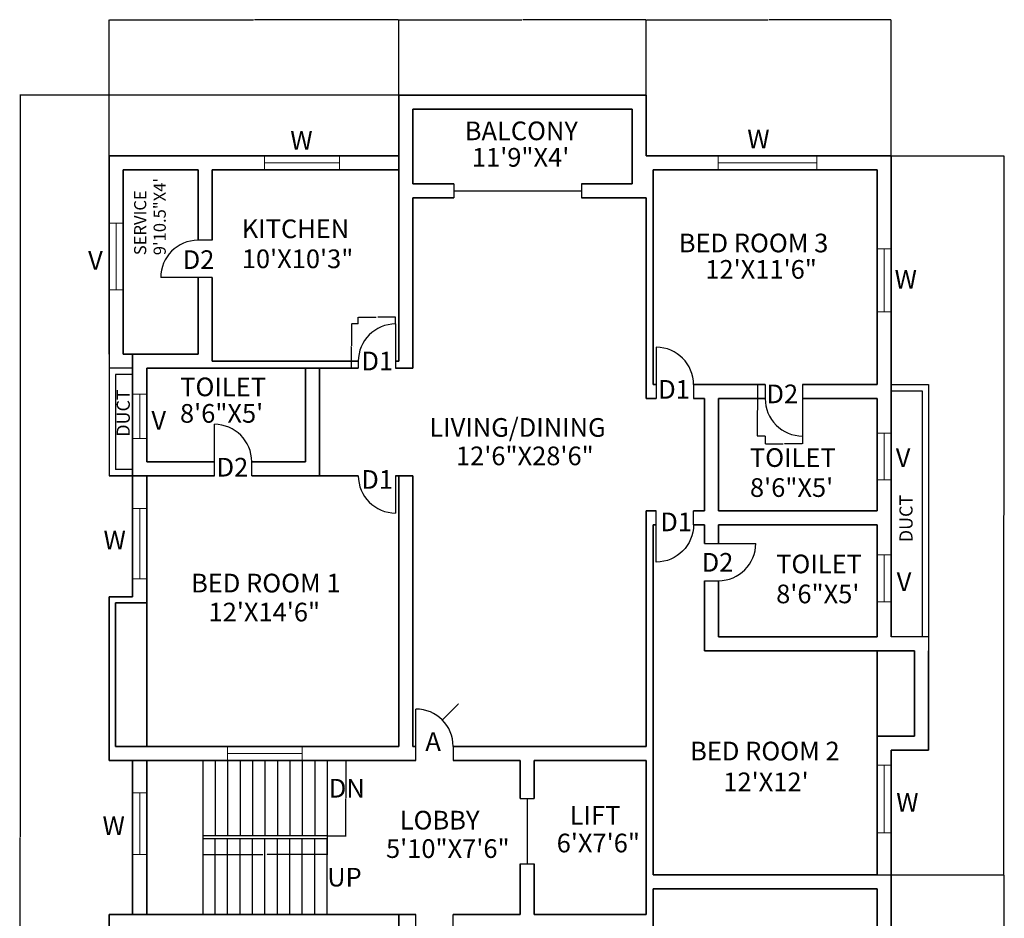
# Model space of a CAD drawing. Units: feet. Extents: x 48598101 to 48598734, y 135188346 to 135189397.
# Tile 2 of 2: x 48598101 to 48598734, y 135188819 to 135189397. Entities that reach past the tile are written whole.
import ezdxf

# ---------------------------------------------------------------- set-up
doc = ezdxf.new("R2010")
doc.units = ezdxf.units.FT
for name, color, linetype, lineweight in [('A-ANNO-DIMS', 2, 'Continuous', 18), ('A-ANNO-TEXT', 7, 'Continuous', 18), ('A-AREA-IDEN', 7, 'Continuous', 18), ('A-DOOR', 3, 'Continuous', 25), ('A-FLOR-SHFT', 7, 'Continuous', 25), ('A-FLOR-STRS', 7, 'Continuous', 25), ('A-GLAZ', 4, 'Continuous', 18), ('A-WALL', 7, 'Continuous', 35)]:
    doc.layers.add(name, color=color, linetype=linetype, lineweight=lineweight)
doc.styles.get("Standard").update_dxf_attribs({"font": 'arial.ttf'})
doc.dimstyles.get("Standard").update_dxf_attribs({"dimtxt": 0.18, "dimasz": 0.18, "dimexe": 0.18, "dimexo": 0.0625, "dimgap": 0.09, "dimtad": 0, "dimtih": 1, "dimtoh": 1, "dimdec": 4, "dimzin": 0, "dimdsep": 46, "dimtxsty": 'Standard', "dimcen": 0.09, "dimadec": 0, "dimazin": 0, "dimtfac": 1, "dimtdec": 4, "dimtofl": 0, "dimtmove": 0, "dimatfit": 3, "dimfxl": 1, "dimtolj": 1, "dimtzin": 0, "dimarcsym": 0})

# ---------------------------------------------------------------- blocks, each defined once
blk = doc.blocks.new('DOOR-D1-KITCHEN')
for p, q in [((24, 28.5), (24, 0)), ((0, 4.5), (0, 0))]:
    blk.add_line(p, q)
blk.add_arc((24, 4.5), 24, 90, 180)
blk = doc.blocks.new('DOOR-D1-BED-SWING')
blk.add_line((24, 24), (24, 0))
blk.add_arc((24, 24), 24, 180, 270)
blk = doc.blocks.new('DOOR-D1-BED-JAMB')
for p, q in [((0, 33), (0, 0)), ((24, 9), (24, 0))]:
    blk.add_line(p, q)
blk.add_arc((0, 9), 24, 0, 90)
blk = doc.blocks.new('DOOR-D2-SINGLE')
for p, q in [((33, 24), (24, 24)), ((33, 0), (0, 0))]:
    blk.add_line(p, q)
blk.add_arc((24, 0), 24, 90, 180)
blk = doc.blocks.new('STAIR-FLIGHT-10-TREAD')
for p, q in [((8, 48.5), (8, 0)), ((16, 48.5), (16, 0)), ((24, 48.5), (24, 0)), ((32, 48.5), (32, 0)), ((40, 48.5), (40, 0)), ((48, 48.5), (48, 0)), ((56, 48.5), (56, 0)), ((64, 48.5), (64, 0)), ((72, 48.5), (72, 0)), ((80, 48.5), (80, 0)), ((80, 0), (0, 0))]:
    blk.add_line(p, q)
blk = doc.blocks.new('SHAFT-VENT-NARROW')
for p, q in [((0, 78), (0, 0)), ((15, 69), (0, 69)), ((15, 65), (4, 65)), ((4, 65), (4, 4)), ((15, 4), (4, 4))]:
    blk.add_line(p, q)
blk = doc.blocks.new('*D7')
at = {"layer": 'A-ANNO-DIMS', "color": 0, "lineweight": -2, "transparency": 16777216}
for p, q in [((48598579.89, 135189162.29), (48598574.83, 135189162.29)), ((48598575.01, 135189162.11), (48598575.01, 135189145.97)), ((48598575.01, 135189129.47), (48598575.01, 135189145.61)), ((48598579.89, 135189129.29), (48598574.83, 135189129.29))]:
    blk.add_line(p, q, dxfattribs=at)
at = {"layer": 'A-ANNO-DIMS', "color": 0, "transparency": 16777216}
for points in [[(48598574.98, 135189162.11), (48598575.04, 135189162.11), (48598575.01, 135189162.29)], [(48598574.98, 135189129.47), (48598575.04, 135189129.47), (48598575.01, 135189129.29)]]:
    blk.add_solid(points, dxfattribs=at)
at = {"layer": 'Defpoints', "color": 0, "transparency": 16777216}
for p in [(48598575.01, 135189162.29), (48598579.96, 135189162.29), (48598579.96, 135189129.29)]:
    blk.add_point(p, dxfattribs=at)
at = {"layer": 'A-ANNO-DIMS', "color": 0, "transparency": 16777216, "insert": (48598575.01, 135189145.79), "char_height": 0.18, "attachment_point": 5}
blk.add_mtext('\\A1;D2 DOOR 33 TYP.', dxfattribs=at)
blk = doc.blocks.new('*D8')
at = {"layer": 'A-ANNO-DIMS', "color": 0, "lineweight": -2, "transparency": 16777216}
for p, q in [((48598579.96, 135189129.23), (48598579.96, 135189124.16)), ((48598603.96, 135189129.23), (48598603.96, 135189124.16)), ((48598580.14, 135189124.34), (48598591.43, 135189124.34)), ((48598603.78, 135189124.34), (48598592.49, 135189124.34))]:
    blk.add_line(p, q, dxfattribs=at)
at = {"layer": 'A-ANNO-DIMS', "color": 0, "transparency": 16777216}
for points in [[(48598580.14, 135189124.37), (48598580.14, 135189124.31), (48598579.96, 135189124.34)], [(48598603.78, 135189124.37), (48598603.78, 135189124.31), (48598603.96, 135189124.34)]]:
    blk.add_solid(points, dxfattribs=at)
at = {"layer": 'Defpoints', "color": 0, "transparency": 16777216}
for p in [(48598579.96, 135189129.29), (48598603.96, 135189129.29), (48598579.96, 135189124.34)]:
    blk.add_point(p, dxfattribs=at)
at = {"layer": 'A-ANNO-DIMS', "color": 0, "transparency": 16777216, "insert": (48598591.96, 135189124.34), "char_height": 0.18, "attachment_point": 5}
blk.add_mtext('\\A1;24 TYP.', dxfattribs=at)
blk = doc.blocks.new('*D11')
at = {"layer": 'A-ANNO-DIMS', "color": 0, "lineweight": -2, "transparency": 16777216}
for p, q in [((48598318.39, 135189201.29), (48598314, 135189201.29)), ((48598314.18, 135189201.11), (48598314.18, 135189187.22)), ((48598314.18, 135189172.97), (48598314.18, 135189186.86)), ((48598318.39, 135189172.79), (48598314, 135189172.79))]:
    blk.add_line(p, q, dxfattribs=at)
at = {"layer": 'A-ANNO-DIMS', "color": 0, "transparency": 16777216}
for points in [[(48598314.15, 135189201.11), (48598314.21, 135189201.11), (48598314.18, 135189201.29)], [(48598314.15, 135189172.97), (48598314.21, 135189172.97), (48598314.18, 135189172.79)]]:
    blk.add_solid(points, dxfattribs=at)
at = {"layer": 'Defpoints', "color": 0, "transparency": 16777216}
for p in [(48598314.18, 135189201.29), (48598318.46, 135189201.29), (48598318.46, 135189172.79)]:
    blk.add_point(p, dxfattribs=at)
at = {"layer": 'A-ANNO-DIMS', "color": 0, "transparency": 16777216, "insert": (48598314.18, 135189187.04), "char_height": 0.18, "attachment_point": 5}
blk.add_mtext('\\A1;D1 KITCHEN 29 TYP.', dxfattribs=at)
blk = doc.blocks.new('*D12')
at = {"layer": 'A-ANNO-DIMS', "color": 0, "lineweight": -2, "transparency": 16777216}
for p, q in [((48598318.46, 135189201.35), (48598318.46, 135189205.75)), ((48598318.64, 135189205.57), (48598329.93, 135189205.57)), ((48598342.28, 135189205.57), (48598330.99, 135189205.57)), ((48598342.46, 135189201.35), (48598342.46, 135189205.75))]:
    blk.add_line(p, q, dxfattribs=at)
at = {"layer": 'A-ANNO-DIMS', "color": 0, "transparency": 16777216}
for points in [[(48598318.64, 135189205.6), (48598318.64, 135189205.54), (48598318.46, 135189205.57)], [(48598342.28, 135189205.6), (48598342.28, 135189205.54), (48598342.46, 135189205.57)]]:
    blk.add_solid(points, dxfattribs=at)
at = {"layer": 'Defpoints', "color": 0, "transparency": 16777216}
for p in [(48598342.46, 135189205.57), (48598318.46, 135189201.29), (48598342.46, 135189201.29)]:
    blk.add_point(p, dxfattribs=at)
at = {"layer": 'A-ANNO-DIMS', "color": 0, "transparency": 16777216, "insert": (48598330.46, 135189205.57), "char_height": 0.18, "attachment_point": 5}
blk.add_mtext('\\A1;24 TYP.', dxfattribs=at)
blk = doc.blocks.new('*D15')
at = {"layer": 'A-ANNO-DIMS', "color": 0, "lineweight": -2, "transparency": 16777216}
for p, q in [((48598218.46, 135188872.23), (48598218.46, 135188860.11)), ((48598298.46, 135188872.23), (48598298.46, 135188860.11)), ((48598218.64, 135188860.29), (48598257.04, 135188860.29)), ((48598298.28, 135188860.29), (48598259.87, 135188860.29))]:
    blk.add_line(p, q, dxfattribs=at)
at = {"layer": 'A-ANNO-DIMS', "color": 0, "transparency": 16777216}
for points in [[(48598218.64, 135188860.32), (48598218.64, 135188860.26), (48598218.46, 135188860.29)], [(48598298.28, 135188860.32), (48598298.28, 135188860.26), (48598298.46, 135188860.29)]]:
    blk.add_solid(points, dxfattribs=at)
at = {"layer": 'Defpoints', "color": 0, "transparency": 16777216}
for p in [(48598218.46, 135188872.29), (48598298.46, 135188872.29), (48598298.46, 135188860.29)]:
    blk.add_point(p, dxfattribs=at)
at = {"layer": 'A-ANNO-DIMS', "color": 0, "transparency": 16777216, "insert": (48598258.46, 135188860.29), "char_height": 0.18, "attachment_point": 5}
blk.add_mtext('\\A1;STAIR FLIGHT 80 TYP.', dxfattribs=at)
blk = doc.blocks.new('*D16')
at = {"layer": 'A-ANNO-DIMS', "color": 0, "lineweight": -2, "transparency": 16777216}
for p, q in [((48598298.52, 135188920.79), (48598310.64, 135188920.79)), ((48598310.46, 135188920.61), (48598310.46, 135188896.72)), ((48598310.46, 135188872.47), (48598310.46, 135188896.36)), ((48598298.52, 135188872.29), (48598310.64, 135188872.29))]:
    blk.add_line(p, q, dxfattribs=at)
at = {"layer": 'A-ANNO-DIMS', "color": 0, "transparency": 16777216}
for points in [[(48598310.43, 135188920.61), (48598310.49, 135188920.61), (48598310.46, 135188920.79)], [(48598310.43, 135188872.47), (48598310.49, 135188872.47), (48598310.46, 135188872.29)]]:
    blk.add_solid(points, dxfattribs=at)
at = {"layer": 'Defpoints', "color": 0, "transparency": 16777216}
for p in [(48598298.46, 135188920.79), (48598310.46, 135188920.79), (48598298.46, 135188872.29)]:
    blk.add_point(p, dxfattribs=at)
at = {"layer": 'A-ANNO-DIMS', "color": 0, "transparency": 16777216, "insert": (48598310.46, 135188896.54), "char_height": 0.18, "attachment_point": 5}
blk.add_mtext('\\A1;49 TYP.', dxfattribs=at)
blk = doc.blocks.new('*D19')
at = {"layer": 'A-ANNO-DIMS', "color": 0, "lineweight": -2, "transparency": 16777216}
for p, q in [((48598503.39, 135189348.29), (48598100.88, 135189348.29)), ((48598101.06, 135189348.11), (48598101.06, 135188871.47)), ((48598101.06, 135188394.47), (48598101.06, 135188871.11)), ((48598353.39, 135188394.29), (48598100.88, 135188394.29))]:
    blk.add_line(p, q, dxfattribs=at)
at = {"layer": 'A-ANNO-DIMS', "color": 0, "transparency": 16777216}
for points in [[(48598101.03, 135189348.11), (48598101.09, 135189348.11), (48598101.06, 135189348.29)], [(48598101.03, 135188394.47), (48598101.09, 135188394.47), (48598101.06, 135188394.29)]]:
    blk.add_solid(points, dxfattribs=at)
at = {"layer": 'Defpoints', "color": 0, "transparency": 16777216}
for p in [(48598503.46, 135189348.29), (48598101.06, 135188394.29), (48598353.46, 135188394.29)]:
    blk.add_point(p, dxfattribs=at)
at = {"layer": 'A-ANNO-DIMS', "color": 0, "transparency": 16777216, "insert": (48598101.06, 135188871.29), "char_height": 0.18, "attachment_point": 5}
blk.add_mtext('\\A1;954', dxfattribs=at)
blk = doc.blocks.new('*D21')
at = {"layer": 'A-ANNO-DIMS', "color": 0, "lineweight": -2, "transparency": 16777216}
for p, q in [((48598158.46, 135189309.35), (48598158.46, 135189396.87)), ((48598158.64, 135189396.69), (48598251.18, 135189396.69)), ((48598344.28, 135189396.69), (48598251.74, 135189396.69)), ((48598344.46, 135189309.35), (48598344.46, 135189396.87))]:
    blk.add_line(p, q, dxfattribs=at)
at = {"layer": 'A-ANNO-DIMS', "color": 0, "transparency": 16777216}
for points in [[(48598158.64, 135189396.72), (48598158.64, 135189396.66), (48598158.46, 135189396.69)], [(48598344.28, 135189396.72), (48598344.28, 135189396.66), (48598344.46, 135189396.69)]]:
    blk.add_solid(points, dxfattribs=at)
at = {"layer": 'Defpoints', "color": 0, "transparency": 16777216}
for p in [(48598344.46, 135189396.69), (48598158.46, 135189309.29), (48598344.46, 135189309.29)]:
    blk.add_point(p, dxfattribs=at)
at = {"layer": 'A-ANNO-DIMS', "color": 0, "transparency": 16777216, "insert": (48598251.46, 135189396.69), "char_height": 0.18, "attachment_point": 5}
blk.add_mtext('\\A1;186', dxfattribs=at)
blk = doc.blocks.new('*D22')
at = {"layer": 'A-ANNO-DIMS', "color": 0, "lineweight": -2, "transparency": 16777216}
for p, q in [((48598344.46, 135189348.35), (48598344.46, 135189396.87)), ((48598344.64, 135189396.69), (48598423.68, 135189396.69)), ((48598503.28, 135189396.69), (48598424.24, 135189396.69)), ((48598503.46, 135189348.35), (48598503.46, 135189396.87))]:
    blk.add_line(p, q, dxfattribs=at)
at = {"layer": 'A-ANNO-DIMS', "color": 0, "transparency": 16777216}
for points in [[(48598344.64, 135189396.72), (48598344.64, 135189396.66), (48598344.46, 135189396.69)], [(48598503.28, 135189396.72), (48598503.28, 135189396.66), (48598503.46, 135189396.69)]]:
    blk.add_solid(points, dxfattribs=at)
at = {"layer": 'Defpoints', "color": 0, "transparency": 16777216}
for p in [(48598503.46, 135189396.69), (48598344.46, 135189348.29), (48598503.46, 135189348.29)]:
    blk.add_point(p, dxfattribs=at)
at = {"layer": 'A-ANNO-DIMS', "color": 0, "transparency": 16777216, "insert": (48598423.96, 135189396.69), "char_height": 0.18, "attachment_point": 5}
blk.add_mtext('\\A1;159', dxfattribs=at)
blk = doc.blocks.new('*D23')
at = {"layer": 'A-ANNO-DIMS', "color": 0, "lineweight": -2, "transparency": 16777216}
for p, q in [((48598503.46, 135189309.35), (48598503.46, 135189396.87)), ((48598503.64, 135189396.69), (48598581.82, 135189396.69)), ((48598660.78, 135189396.69), (48598582.59, 135189396.69)), ((48598660.96, 135189309.35), (48598660.96, 135189396.87))]:
    blk.add_line(p, q, dxfattribs=at)
at = {"layer": 'A-ANNO-DIMS', "color": 0, "transparency": 16777216}
for points in [[(48598503.64, 135189396.72), (48598503.64, 135189396.66), (48598503.46, 135189396.69)], [(48598660.78, 135189396.72), (48598660.78, 135189396.66), (48598660.96, 135189396.69)]]:
    blk.add_solid(points, dxfattribs=at)
at = {"layer": 'Defpoints', "color": 0, "transparency": 16777216}
for p in [(48598660.96, 135189396.69), (48598503.46, 135189309.29), (48598660.96, 135189309.29)]:
    blk.add_point(p, dxfattribs=at)
at = {"layer": 'A-ANNO-DIMS', "color": 0, "transparency": 16777216, "insert": (48598582.21, 135189396.69), "char_height": 0.18, "attachment_point": 5}
blk.add_mtext('\\A1;157.5', dxfattribs=at)
blk = doc.blocks.new('*D24')
at = {"layer": 'A-ANNO-DIMS', "color": 0, "lineweight": -2, "transparency": 16777216}
for p, q in [((48598661.02, 135189309.29), (48598733.54, 135189309.29)), ((48598733.36, 135189309.11), (48598733.36, 135189078.47)), ((48598733.36, 135188847.47), (48598733.36, 135189078.11)), ((48598652.02, 135188847.29), (48598733.54, 135188847.29))]:
    blk.add_line(p, q, dxfattribs=at)
at = {"layer": 'A-ANNO-DIMS', "color": 0, "transparency": 16777216}
for points in [[(48598733.33, 135189309.11), (48598733.39, 135189309.11), (48598733.36, 135189309.29)], [(48598733.33, 135188847.47), (48598733.39, 135188847.47), (48598733.36, 135188847.29)]]:
    blk.add_solid(points, dxfattribs=at)
at = {"layer": 'Defpoints', "color": 0, "transparency": 16777216}
for p in [(48598660.96, 135189309.29), (48598651.96, 135188847.29), (48598733.36, 135188847.29)]:
    blk.add_point(p, dxfattribs=at)
at = {"layer": 'A-ANNO-DIMS', "color": 0, "transparency": 16777216, "insert": (48598733.36, 135189078.29), "char_height": 0.18, "attachment_point": 5}
blk.add_mtext('\\A1;462', dxfattribs=at)
blk = doc.blocks.new('*D25')
at = {"layer": 'A-ANNO-DIMS', "color": 0, "lineweight": -2, "transparency": 16777216}
for p, q in [((48598652.02, 135188847.29), (48598733.54, 135188847.29)), ((48598733.36, 135188847.11), (48598733.36, 135188630.72)), ((48598733.36, 135188413.97), (48598733.36, 135188630.36)), ((48598661.02, 135188413.79), (48598733.54, 135188413.79))]:
    blk.add_line(p, q, dxfattribs=at)
at = {"layer": 'A-ANNO-DIMS', "color": 0, "transparency": 16777216}
for points in [[(48598733.33, 135188847.11), (48598733.39, 135188847.11), (48598733.36, 135188847.29)], [(48598733.33, 135188413.97), (48598733.39, 135188413.97), (48598733.36, 135188413.79)]]:
    blk.add_solid(points, dxfattribs=at)
at = {"layer": 'Defpoints', "color": 0, "transparency": 16777216}
for p in [(48598651.96, 135188847.29), (48598660.96, 135188413.79), (48598733.36, 135188413.79)]:
    blk.add_point(p, dxfattribs=at)
at = {"layer": 'A-ANNO-DIMS', "color": 0, "transparency": 16777216, "insert": (48598733.36, 135188630.54), "char_height": 0.18, "attachment_point": 5}
blk.add_mtext('\\A1;433.5', dxfattribs=at)
blk = doc.blocks.new('*D26')
at = {"layer": 'A-ANNO-DIMS', "color": 0, "lineweight": -2, "transparency": 16777216}
for p, q in [((48598382.61, 135188956.94), (48598372.55, 135188946.89)), ((48598382.79, 135188956.94), (48598382.61, 135188956.94)), ((48598355.37, 135188929.79), (48598355.55, 135188929.79)), ((48598355.46, 135188929.7), (48598355.46, 135188929.88))]:
    blk.add_line(p, q, dxfattribs=at)
at = {"layer": 'A-ANNO-DIMS', "color": 0, "transparency": 16777216}
blk.add_solid([(48598372.53, 135188946.91), (48598372.58, 135188946.87), (48598372.43, 135188946.76)], dxfattribs=at)
at = {"layer": 'Defpoints', "color": 0, "transparency": 16777216}
for p in [(48598372.43, 135188946.76), (48598355.46, 135188929.79)]:
    blk.add_point(p, dxfattribs=at)
at = {"layer": 'A-ANNO-DIMS', "color": 0, "transparency": 16777216, "insert": (48598383.35, 135188956.94), "char_height": 0.18, "attachment_point": 5}
blk.add_mtext('\\A1;16X R24', dxfattribs=at)

msp = doc.modelspace()

# ---------------------------------------------------------------- linework, layer by layer
at = {"layer": 'A-DOOR'}
for p, q in [((48598379.79, 135189291.29), (48598379.79, 135189282.29)), ((48598379.79, 135189286.79), (48598462.02, 135189286.79)), ((48598462.02, 135189291.29), (48598462.02, 135189282.29)), ((48598342.46, 135189201.29), (48598342.46, 135189201.29)), ((48598355.46, 135188920.79), (48598355.46, 135188953.79)), ((48598379.46, 135188929.79), (48598379.46, 135188920.79)), ((48598422.46, 135188896.4), (48598431.46, 135188896.4)), ((48598426.96, 135188896.4), (48598426.96, 135188854.27)), ((48598422.46, 135188854.27), (48598431.46, 135188854.27)), ((48598355.46, 135188802.29), (48598355.46, 135188821.79)), ((48598379.46, 135188812.79), (48598379.46, 135188821.79))]:
    msp.add_line(p, q, dxfattribs=at)
msp.add_arc((48598355.46, 135188929.79), 24, 0, 90, dxfattribs=at)
at = {"layer": 'A-FLOR-SHFT'}
for p, q in [((48598684.96, 135189000.29), (48598660.96, 135189000.29)), ((48598684.96, 135188991.93), (48598684.96, 135188991.29))]:
    msp.add_line(p, q, dxfattribs=at)
for points in [[(48598660.96, 135189162.29), (48598684.96, 135189162.29), (48598684.96, 135188991.93)], [(48598660.96, 135189158.29), (48598680.96, 135189158.29), (48598680.96, 135189000.29)]]:
    msp.add_lwpolyline(points, dxfattribs=at)
at = {"layer": 'A-FLOR-STRS'}
msp.add_line((48598218.46, 135188920.79), (48598218.46, 135188821.79), dxfattribs=at)
at = {"layer": 'A-GLAZ'}
for p, q in [((48598258.23, 135189309.29), (48598258.23, 135189300.29)), ((48598306.31, 135189309.29), (48598306.31, 135189300.29)), ((48598549.7, 135189309.29), (48598549.7, 135189300.29)), ((48598613.08, 135189309.29), (48598613.08, 135189300.29)), ((48598258.23, 135189304.79), (48598306.31, 135189304.79)), ((48598549.7, 135189304.79), (48598613.08, 135189304.79)), ((48598158.46, 135189266.19), (48598167.46, 135189266.19)), ((48598162.96, 135189266.19), (48598162.96, 135189223.24)), ((48598651.96, 135189249.51), (48598660.96, 135189249.51)), ((48598656.46, 135189249.51), (48598656.46, 135189209.05)), ((48598158.46, 135189223.24), (48598167.46, 135189223.24)), ((48598651.96, 135189209.05), (48598660.96, 135189209.05)), ((48598173.46, 135189156.24), (48598182.46, 135189156.24)), ((48598177.96, 135189156.24), (48598177.96, 135189127.77)), ((48598651.96, 135189131.15), (48598660.96, 135189131.15)), ((48598656.46, 135189131.15), (48598656.46, 135189101.15)), ((48598173.46, 135189127.77), (48598182.46, 135189127.77)), ((48598651.96, 135189101.15), (48598660.96, 135189101.15)), ((48598173.46, 135189082.74), (48598182.46, 135189082.74)), ((48598177.96, 135189082.74), (48598177.96, 135189037.54)), ((48598651.96, 135189052.92), (48598660.96, 135189052.92)), ((48598656.46, 135189052.92), (48598656.46, 135189022.73)), ((48598173.46, 135189037.54), (48598182.46, 135189037.54)), ((48598651.96, 135189022.73), (48598660.96, 135189022.73)), ((48598234.46, 135188920.79), (48598234.46, 135188929.79)), ((48598282.46, 135188920.79), (48598282.46, 135188929.79)), ((48598234.46, 135188925.29), (48598282.46, 135188925.29)), ((48598651.96, 135188917.66), (48598660.96, 135188917.66)), ((48598656.46, 135188917.66), (48598656.46, 135188874.32)), ((48598173.46, 135188900.02), (48598182.46, 135188900.02)), ((48598177.96, 135188900.02), (48598177.96, 135188860.2)), ((48598651.96, 135188874.32), (48598660.96, 135188874.32)), ((48598173.46, 135188860.2), (48598182.46, 135188860.2))]:
    msp.add_line(p, q, dxfattribs=at)
at = {"layer": 'A-WALL'}
for p, q in [((48598344.46, 135189291.29), (48598344.46, 135189348.29)), ((48598344.46, 135189348.29), (48598503.46, 135189348.29)), ((48598503.46, 135189348.29), (48598503.46, 135189309.29)), ((48598353.46, 135189291.29), (48598353.46, 135189339.29)), ((48598353.46, 135189339.29), (48598494.46, 135189339.29)), ((48598494.46, 135189339.29), (48598494.46, 135189291.29)), ((48598158.46, 135189309.29), (48598344.46, 135189309.29)), ((48598158.46, 135189181.79), (48598158.46, 135189309.29)), ((48598224.46, 135189309.29), (48598344.46, 135189309.29)), ((48598503.46, 135189309.29), (48598660.96, 135189309.29)), ((48598660.96, 135189309.29), (48598660.96, 135189000.29)), ((48598167.46, 135189300.29), (48598215.46, 135189300.29)), ((48598167.46, 135189181.79), (48598167.46, 135189300.29)), ((48598215.46, 135189300.29), (48598215.46, 135189255.07)), ((48598224.46, 135189300.29), (48598224.46, 135189255.07)), ((48598224.46, 135189300.29), (48598344.46, 135189300.29)), ((48598344.46, 135189300.29), (48598344.46, 135189177.29)), ((48598507.96, 135189300.29), (48598507.96, 135189162.29)), ((48598507.96, 135189300.29), (48598651.96, 135189300.29)), ((48598651.96, 135189300.29), (48598651.96, 135189162.29)), ((48598353.46, 135189291.29), (48598379.79, 135189291.29)), ((48598462.02, 135189291.29), (48598494.46, 135189291.29)), ((48598353.46, 135189282.29), (48598379.79, 135189282.29)), ((48598353.46, 135189282.29), (48598353.46, 135189177.29)), ((48598353.46, 135189172.79), (48598353.46, 135189282.29)), ((48598462.02, 135189282.29), (48598503.46, 135189282.29)), ((48598503.46, 135189282.29), (48598503.46, 135189153.29)), ((48598215.46, 135189231.07), (48598215.46, 135189181.79)), ((48598224.46, 135189231.07), (48598224.46, 135189177.29)), ((48598215.46, 135189181.79), (48598167.46, 135189181.79)), ((48598173.46, 135189112.79), (48598173.46, 135189181.79)), ((48598215.46, 135189172.79), (48598182.46, 135189172.79)), ((48598182.46, 135189112.79), (48598182.46, 135189172.79)), ((48598215.46, 135189172.79), (48598318.46, 135189172.79)), ((48598318.46, 135189177.29), (48598224.46, 135189177.29)), ((48598284.46, 135189172.79), (48598284.46, 135189112.79)), ((48598293.46, 135189172.79), (48598293.46, 135189103.79)), ((48598344.46, 135189177.29), (48598342.46, 135189177.29)), ((48598342.46, 135189172.79), (48598353.46, 135189172.79)), ((48598509.96, 135189162.29), (48598507.96, 135189162.29)), ((48598579.96, 135189162.29), (48598533.96, 135189162.29)), ((48598651.96, 135189162.29), (48598603.96, 135189162.29)), ((48598509.96, 135189153.29), (48598503.46, 135189153.29)), ((48598540.96, 135189153.29), (48598533.96, 135189153.29)), ((48598540.96, 135189081.29), (48598540.96, 135189153.29)), ((48598549.96, 135189081.29), (48598549.96, 135189153.29)), ((48598579.96, 135189153.29), (48598549.96, 135189153.29)), ((48598651.96, 135189153.29), (48598603.96, 135189153.29)), ((48598651.96, 135189153.29), (48598651.96, 135189081.29)), ((48598660.96, 135189153.29), (48598660.96, 135189081.29)), ((48598173.46, 135189112.79), (48598173.46, 135189025.97)), ((48598225.96, 135189112.79), (48598182.46, 135189112.79)), ((48598284.46, 135189112.79), (48598249.96, 135189112.79)), ((48598225.96, 135189103.79), (48598158.46, 135189103.79)), ((48598182.46, 135189103.79), (48598182.46, 135188929.79)), ((48598293.46, 135189103.79), (48598249.96, 135189103.79)), ((48598293.46, 135189103.79), (48598318.46, 135189103.79)), ((48598342.46, 135189103.79), (48598353.46, 135189103.79)), ((48598344.46, 135189103.79), (48598344.46, 135188929.79)), ((48598353.46, 135188929.79), (48598353.46, 135189103.79)), ((48598549.96, 135189081.29), (48598549.96, 135189096.29)), ((48598503.46, 135189081.29), (48598503.46, 135188940.29)), ((48598509.96, 135189081.29), (48598503.46, 135189081.29)), ((48598540.96, 135189081.29), (48598533.96, 135189081.29)), ((48598651.96, 135189081.29), (48598549.96, 135189081.29)), ((48598507.96, 135189072.29), (48598507.96, 135188940.29)), ((48598509.96, 135189072.29), (48598507.96, 135189072.29)), ((48598540.96, 135189072.29), (48598533.96, 135189072.29)), ((48598540.96, 135189060.29), (48598540.96, 135189072.29)), ((48598540.96, 135189060.29), (48598540.96, 135189072.29)), ((48598651.96, 135189072.29), (48598549.96, 135189072.29)), ((48598549.96, 135189060.29), (48598549.96, 135189072.29)), ((48598651.96, 135189072.29), (48598651.96, 135189000.29)), ((48598660.96, 135189072.29), (48598660.96, 135189000.29)), ((48598540.96, 135188991.29), (48598540.96, 135189036.29)), ((48598540.96, 135189000.29), (48598540.96, 135189036.29)), ((48598549.96, 135189000.29), (48598549.96, 135189036.29)), ((48598158.46, 135189025.97), (48598158.46, 135188920.79)), ((48598158.46, 135189025.97), (48598173.46, 135189025.97)), ((48598162.46, 135189021.97), (48598182.46, 135189021.97)), ((48598162.46, 135189021.97), (48598162.46, 135188929.79)), ((48598555.96, 135189000.29), (48598549.96, 135189000.29)), ((48598651.96, 135189000.29), (48598555.96, 135189000.29)), ((48598507.96, 135188847.29), (48598507.96, 135188991.29)), ((48598675.96, 135188991.29), (48598540.96, 135188991.29)), ((48598651.96, 135188991.29), (48598651.96, 135188847.29)), ((48598675.96, 135188991.29), (48598675.96, 135188936.31)), ((48598684.96, 135188991.29), (48598684.96, 135188927.31)), ((48598503.46, 135188940.29), (48598503.46, 135188929.79)), ((48598675.96, 135188936.31), (48598651.96, 135188936.31)), ((48598162.46, 135188929.79), (48598344.46, 135188929.79)), ((48598353.46, 135188929.79), (48598355.46, 135188929.79)), ((48598379.46, 135188929.79), (48598503.46, 135188929.79)), ((48598684.96, 135188927.31), (48598660.96, 135188927.31)), ((48598660.96, 135188927.31), (48598660.96, 135188838.29)), ((48598660.96, 135188927.31), (48598660.96, 135188838.29)), ((48598158.46, 135188920.79), (48598355.46, 135188920.79)), ((48598173.46, 135188920.79), (48598173.46, 135188821.79)), ((48598182.46, 135188920.79), (48598182.46, 135188821.79)), ((48598379.46, 135188920.79), (48598422.46, 135188920.79)), ((48598422.46, 135188896.4), (48598422.46, 135188920.79)), ((48598431.46, 135188920.79), (48598503.46, 135188920.79)), ((48598431.46, 135188896.4), (48598431.46, 135188920.79)), ((48598503.46, 135188920.79), (48598503.46, 135188821.79)), ((48598422.46, 135188821.79), (48598422.46, 135188854.27)), ((48598431.46, 135188821.79), (48598431.46, 135188854.27)), ((48598651.96, 135188847.29), (48598507.96, 135188847.29)), ((48598651.96, 135188838.29), (48598507.96, 135188838.29)), ((48598507.96, 135188613.29), (48598507.96, 135188838.29)), ((48598651.96, 135188838.29), (48598507.96, 135188838.29)), ((48598651.96, 135188613.29), (48598651.96, 135188838.29)), ((48598660.96, 135188758.27), (48598660.96, 135188838.29)), ((48598165.96, 135188821.79), (48598158.46, 135188821.79)), ((48598158.46, 135188821.79), (48598344.46, 135188821.79)), ((48598158.46, 135188694.29), (48598158.46, 135188821.79)), ((48598344.46, 135188821.79), (48598173.46, 135188821.79)), ((48598224.46, 135188821.79), (48598344.46, 135188821.79)), ((48598344.46, 135188803.79), (48598344.46, 135188821.79)), ((48598355.46, 135188821.79), (48598344.46, 135188821.79)), ((48598422.46, 135188821.79), (48598379.46, 135188821.79)), ((48598503.46, 135188821.79), (48598431.46, 135188821.79))]:
    msp.add_line(p, q, dxfattribs=at)

# ---------------------------------------------------------------- block references
at = {"layer": 'A-DOOR'}
for name, p in [('DOOR-D2-SINGLE', (48598191.46, 135189231.07)), ('DOOR-D1-KITCHEN', (48598318.46, 135189172.79)), ('DOOR-D1-BED-JAMB', (48598509.96, 135189153.29)), ('DOOR-D1-BED-SWING', (48598318.46, 135189079.79))]:
    msp.add_blockref(name, p, dxfattribs=at)
for p, rotation in [((48598603.96, 135189129.29), 90.00000021460632), ((48598225.96, 135189136.79), 270.0000001790853), ((48598573.96, 135189060.29), 180)]:
    msp.add_blockref('DOOR-D2-SINGLE', p, dxfattribs=dict(at, rotation=rotation))
at = {"layer": 'A-DOOR', "extrusion": (0, 0, -1), "zscale": -1, "rotation": 180}
msp.add_blockref('DOOR-D1-BED-JAMB', (-48598509.96, 135189081.29), dxfattribs=at)
at = {"layer": 'A-FLOR-SHFT'}
msp.add_blockref('SHAFT-VENT-NARROW', (48598158.46, 135189103.79), dxfattribs=at)
at = {"layer": 'A-FLOR-STRS'}
msp.add_blockref('STAIR-FLIGHT-10-TREAD', (48598218.46, 135188872.29), dxfattribs=at)
at = {"layer": 'A-FLOR-STRS', "extrusion": (0, 0, -1), "zscale": -1, "rotation": 180}
msp.add_blockref('STAIR-FLIGHT-10-TREAD', (-48598218.46, 135188870.29), dxfattribs=at)

# ---------------------------------------------------------------- texts
at = {"layer": 'A-ANNO-DIMS'}
for s, p in [('11\'9"X4\'', (48598391.5, 135189302.41)), ('10\'X10\'3"', (48598243.59, 135189237.17)), ('12\'X11\'6"', (48598541.52, 135189230.38)), ('8\'6"X5\'', (48598203.86, 135189137.82)), ('12\'6"X28\'6"', (48598381.25, 135189110.51)), ('8\'6"X5\'', (48598570.19, 135189090.15)), ('8\'6"X5\'', (48598587.03, 135189021.78)), ('12\'X14\'6"', (48598222.23, 135189010.11)), ("12'X12'", (48598553.07, 135188900.99)), ('5\'10"X7\'6"', (48598336.28, 135188858.1)), ('6\'X7\'6"', (48598445.98, 135188861.69))]:
    msp.add_text(s, height=12, dxfattribs=at).set_placement(p)
msp.add_text('9\'10.5"X4\'', height=7.81, rotation=90, dxfattribs=at).set_placement((48598194.74, 135189245.5))
at = {"layer": 'A-ANNO-TEXT'}
for s, p in [('W', (48598274.75, 135189313.33)), ('W', (48598568.46, 135189314.23)), ('D2', (48598205.61, 135189236.64)), ('V', (48598144.83, 135189236.15)), ('W', (48598663.14, 135189224.08)), ('D1', (48598320.51, 135189171.49)), ('D1', (48598511.23, 135189153.26)), ('D2', (48598580.81, 135189150.36)), ('V', (48598185.49, 135189133.35)), ('V', (48598663.89, 135189109.42)), ('D2', (48598227.39, 135189103.23)), ('D1', (48598320.38, 135189095.35)), ('D1', (48598512.55, 135189068.09)), ('W', (48598154.72, 135189056.48)), ('D2', (48598539.16, 135189042.09)), ('V', (48598664.51, 135189029.58)), ('DN', (48598299.53, 135188896.89)), ('W', (48598664.17, 135188887.88)), ('W', (48598154.07, 135188872.85)), ('UP', (48598298.5, 135188839.73))]:
    msp.add_text(s, height=12, dxfattribs=at).set_placement(p)
at = {"layer": 'A-AREA-IDEN'}
for s, p in [('BALCONY', (48598386.91, 135189319.41)), ('KITCHEN', (48598243.59, 135189256.45)), ('BED ROOM 3', (48598524.48, 135189247.35)), ('TOILET', (48598204.05, 135189154.86)), ('LIVING/DINING', (48598364.15, 135189128.78)), ('TOILET', (48598570.19, 135189109.42)), ('TOILET', (48598587.03, 135189041.05)), ('BED ROOM 1', (48598211.02, 135189028.76)), ('A', (48598361.58, 135188926.92)), ('BED ROOM 2', (48598531.77, 135188920.8)), ('LOBBY', (48598345.12, 135188876.37)), ('LIFT', (48598454.35, 135188879.57))]:
    msp.add_text(s, height=12, dxfattribs=at).set_placement(p)
for s, height, p in [('SERVICE', 7.81, (48598182.2, 135189245.5)), ('DUCT', 8.447, (48598171.63, 135189128.8)), ('DUCT', 8.447, (48598674.71, 135189061))]:
    msp.add_text(s, height=height, rotation=90, dxfattribs=at).set_placement(p)

# ---------------------------------------------------------------- dimensions: what is measured, and where the dimension line sits
at = {"layer": 'A-ANNO-DIMS'}
for base, p1, p2, override, picture, middle in [((48598344.46, 135189396.69), (48598158.46, 135189309.29), (48598344.46, 135189309.29), {"dimdec": 0, "dimlfac": 1, "dimrnd": 0, "dimzin": 0, "dimdsep": 46, "dimlunit": 2}, '*D21', (48598251.46, 135189396.69)), ((48598503.46, 135189396.69), (48598344.46, 135189348.29), (48598503.46, 135189348.29), {"dimdec": 0, "dimlfac": 1, "dimrnd": 0, "dimzin": 0, "dimdsep": 46, "dimlunit": 2}, '*D22', (48598423.96, 135189396.69)), ((48598660.96, 135189396.69), (48598503.46, 135189309.29), (48598660.96, 135189309.29), {"dimdec": 1, "dimlfac": 1, "dimrnd": 0, "dimzin": 0, "dimdsep": 46, "dimlunit": 2}, '*D23', (48598582.21, 135189396.69))]:
    dim = msp.add_linear_dim(base=base, p1=p1, p2=p2, dimstyle='Standard', override=override, dxfattribs=at)
    dim.commit()
    dim.dimension.update_dxf_attribs({"geometry": picture, "text_midpoint": middle})
for base, p1, p2, override, picture, middle in [((48598101.06, 135188394.29), (48598503.46, 135189348.29), (48598353.46, 135188394.29), {"dimdec": 0, "dimlfac": 1, "dimrnd": 0, "dimzin": 0, "dimdsep": 46, "dimlunit": 2}, '*D19', (48598101.06, 135188871.29)), ((48598733.36, 135188847.29), (48598660.96, 135189309.29), (48598651.96, 135188847.29), {"dimdec": 0, "dimlfac": 1, "dimrnd": 0, "dimzin": 0, "dimdsep": 46, "dimlunit": 2}, '*D24', (48598733.36, 135189078.29)), ((48598733.36, 135188413.79), (48598651.96, 135188847.29), (48598660.96, 135188413.79), {"dimdec": 1, "dimlfac": 1, "dimrnd": 0, "dimzin": 0, "dimdsep": 46, "dimlunit": 2}, '*D25', (48598733.36, 135188630.54))]:
    dim = msp.add_linear_dim(base=base, p1=p1, p2=p2, angle=90, dimstyle='Standard', override=override, dxfattribs=at)
    dim.commit()
    dim.dimension.update_dxf_attribs({"geometry": picture, "text_midpoint": middle})
for base, p1, p2, text, picture, middle in [((48598342.46, 135189205.57), (48598318.46, 135189201.29), (48598342.46, 135189201.29), '<> TYP.', '*D12', (48598330.46, 135189205.57)), ((48598298.46, 135188860.29), (48598218.46, 135188872.29), (48598298.46, 135188872.29), 'STAIR FLIGHT <> TYP.', '*D15', (48598258.46, 135188860.29))]:
    dim = msp.add_linear_dim(base=base, p1=p1, p2=p2, text=text, dimstyle='Standard', override={"dimdec": 0, "dimlfac": 1, "dimrnd": 0, "dimzin": 0, "dimdsep": 46, "dimlunit": 2}, dxfattribs=at)
    dim.commit()
    dim.dimension.update_dxf_attribs({"geometry": picture, "text_midpoint": middle})
for base, p1, p2, angle, text, picture, middle in [((48598314.18104501, 135189201.29038319), (48598318.45604498, 135189172.7903831), (48598318.45604498, 135189201.2903831), 90, 'D1 KITCHEN <> TYP.', '*D11', (48598314.18104505, 135189187.0403831)), ((48598575.01, 135189162.29), (48598579.96, 135189129.29), (48598579.96, 135189162.29), 90, 'D2 DOOR <> TYP.', '*D7', (48598575.01, 135189145.79)), ((48598579.96, 135189124.34), (48598603.96, 135189129.29), (48598579.96, 135189129.29), 180, '<> TYP.', '*D8', (48598591.96, 135189124.34)), ((48598310.45604501, 135188920.79038319), (48598298.45604498, 135188872.2903831), (48598298.45604498, 135188920.7903831), 90, '<> TYP.', '*D16', (48598310.45604504, 135188896.5403831))]:
    dim = msp.add_linear_dim(base=base, p1=p1, p2=p2, angle=angle, text=text, dimstyle='Standard', override={"dimdec": 0, "dimlfac": 1, "dimrnd": 0, "dimzin": 0, "dimdsep": 46, "dimlunit": 2}, dxfattribs=at)
    dim.commit()
    dim.dimension.update_dxf_attribs({"geometry": picture, "text_midpoint": middle})
dim = msp.add_radius_dim(center=(48598355.46, 135188929.79), mpoint=(48598372.43, 135188946.76), text='16X <>', dimstyle='Standard', override={"dimdec": 0, "dimlfac": 1, "dimrnd": 0, "dimzin": 0, "dimdsep": 46, "dimlunit": 2}, dxfattribs=at)
dim.commit()
dim.dimension.update_dxf_attribs({"geometry": '*D26', "text_midpoint": (48598383.35, 135188956.94), "dimtype": 164})

doc.saveas('drawing.dxf')
